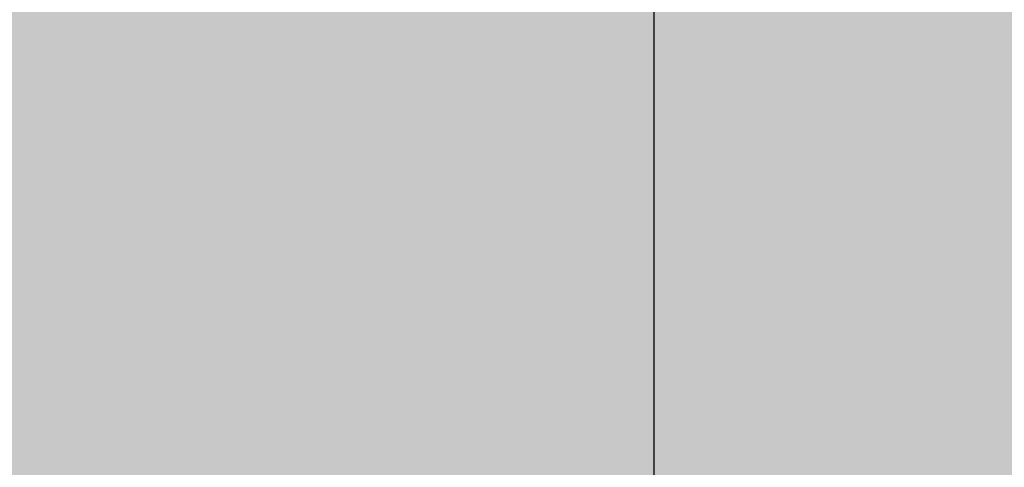
# Model space of a CAD drawing. Units: inches. Extents: x 2083 to 3317, y 1141 to 2115.
# Tile 46 of 256: x 2237.106 to 2238.294, y 1477.116 to 1477.656. Entities that reach past the tile are written whole.
import ezdxf

# ---------------------------------------------------------------- set-up
doc = ezdxf.new("R2010")
doc.units = ezdxf.units.IN
doc.layers.add('A-ANNO-DIMS', color=2, linetype='Continuous', lineweight=18)
doc.layers.add('A-WALL-PATT', color=251, linetype='Continuous', lineweight=13, true_color=0x636466)
doc.styles.get("Standard").update_dxf_attribs({"font": 'arial.ttf'})
doc.dimstyles.new('ISO-25', dxfattribs={"dimtxt": 12, "dimasz": 12, "dimexe": 1.25, "dimexo": 0.625, "dimtad": 1, "dimlunit": 3, "dimtxsty": 'Standard', "dimcen": 2.5, "dimadec": 0, "dimazin": 0, "dimtfac": 1, "dimtmove": 0, "dimatfit": 3, "dimfxl": 1, "dimarcsym": 0})

# ---------------------------------------------------------------- blocks, each defined once
blk = doc.blocks.new('*D30')
at = {"layer": 'A-ANNO-DIMS', "color": 0, "lineweight": -2, "transparency": 16777216}
for p, q in [((2240.0179, 1445.2738), (2240.0179, 1448.0455)), ((2254.3293, 1445.2738), (2254.3293, 1448.0455)), ((2228.0179, 1446.7955), (2216.0179, 1446.7955)), ((2240.0179, 1446.7955), (2254.3293, 1446.7955)), ((2266.3293, 1446.7955), (2413.7649, 1446.7955))]:
    blk.add_line(p, q, dxfattribs=at)
at = {"layer": 'A-ANNO-DIMS', "color": 0, "transparency": 16777216}
for points in [[(2228.0179, 1448.7955), (2228.0179, 1444.7955), (2240.0179, 1446.7955)], [(2266.3293, 1448.7955), (2266.3293, 1444.7955), (2254.3293, 1446.7955)]]:
    blk.add_solid(points, dxfattribs=at)
at = {"layer": 'Defpoints', "color": 0, "transparency": 16777216}
for p in [(2254.3293, 1446.7955), (2240.0179, 1444.6488), (2254.3293, 1444.6488)]:
    blk.add_point(p, dxfattribs=at)
at = {"layer": 'A-ANNO-DIMS', "color": 0, "transparency": 16777216, "insert": (2346.0471, 1453.6252), "char_height": 12, "attachment_point": 5}
blk.add_mtext('WC 1\'-2 1/2" TYP.', dxfattribs=at)
blk = doc.blocks.new('*D31')
at = {"layer": 'A-ANNO-DIMS', "color": 0, "lineweight": -2, "transparency": 16777216}
for p, q in [((2237.8711, 1456.6488), (2237.8711, 1541.9152)), ((2239.3929, 1444.6488), (2236.6211, 1444.6488)), ((2237.8711, 1431.5475), (2237.8711, 1444.6488)), ((2239.3929, 1431.5475), (2236.6211, 1431.5475)), ((2237.8711, 1419.5475), (2237.8711, 1407.5475))]:
    blk.add_line(p, q, dxfattribs=at)
at = {"layer": 'A-ANNO-DIMS', "color": 0, "transparency": 16777216}
for points in [[(2235.8711, 1456.6488), (2239.8711, 1456.6488), (2237.8711, 1444.6488)], [(2235.8711, 1419.5475), (2239.8711, 1419.5475), (2237.8711, 1431.5475)]]:
    blk.add_solid(points, dxfattribs=at)
at = {"layer": 'Defpoints', "color": 0, "transparency": 16777216}
for p in [(2237.8711, 1444.6488), (2240.0179, 1444.6488), (2240.0179, 1431.5475)]:
    blk.add_point(p, dxfattribs=at)
at = {"layer": 'A-ANNO-DIMS', "color": 0, "transparency": 16777216, "insert": (2231.2175, 1505.282), "char_height": 12, "attachment_point": 5, "rotation": 90}
blk.add_mtext('1\'-1" TYP.', dxfattribs=at)
blk = doc.blocks.new('*D62')
at = {"layer": 'A-ANNO-DIMS', "color": 0, "lineweight": -2, "transparency": 16777216}
for p, q in [((2235.9598, 1469.3864), (2235.9598, 1522.3614)), ((2379.9598, 1469.3864), (2379.9598, 1522.3614)), ((2247.9598, 1521.1114), (2367.9598, 1521.1114))]:
    blk.add_line(p, q, dxfattribs=at)
at = {"layer": 'A-ANNO-DIMS', "color": 0, "transparency": 16777216}
for points in [[(2247.9598, 1523.1114), (2247.9598, 1519.1114), (2235.9598, 1521.1114)], [(2367.9598, 1523.1114), (2367.9598, 1519.1114), (2379.9598, 1521.1114)]]:
    blk.add_solid(points, dxfattribs=at)
at = {"layer": 'Defpoints', "color": 0, "transparency": 16777216}
for p in [(2379.9598, 1521.1114), (2235.9598, 1468.7614), (2379.9598, 1468.7614)]:
    blk.add_point(p, dxfattribs=at)
at = {"layer": 'A-ANNO-DIMS', "color": 0, "transparency": 16777216, "insert": (2307.9598, 1527.8632), "char_height": 12, "attachment_point": 5}
blk.add_mtext('12\'-0"', dxfattribs=at)

msp = doc.modelspace()

# ---------------------------------------------------------------- hatches: boundary and pattern name
at = {"layer": 'A-WALL-PATT'}
h = msp.add_hatch(color=256, dxfattribs=at)
h.dxf.hatch_style = 1
h.paths.add_polyline_path([(3126.9598, 2020.7614), (2748.9598, 2020.7614), (2604.9598, 2020.7614), (2226.9598, 2020.7614), (2226.9598, 1702.7614), (2466.9598, 1702.7614), (2466.9598, 1582.7614), (2418.9598, 1582.7614), (2418.9598, 1477.7614), (2226.9598, 1477.7614), (2226.9598, 1263.2614), (2544.9598, 1263.2614), (2544.9598, 1411.7614), (2604.9598, 1411.7614), (2685.9598, 1411.7614), (2685.9598, 1420.7614), (2604.9598, 1420.7614), (2604.9598, 1573.7614), (2604.9598, 1702.7614), (2604.9598, 2011.7614), (2748.9598, 2011.7614), (2748.9598, 1702.7614), (2862.9598, 1702.7614), (2862.9598, 1621.7614), (2871.9598, 1621.7614), (2871.9598, 1702.7614), (2883.9598, 1702.7614), (2883.9598, 1706.9395, -0.026459), (2883.9598, 1711.7614), (2757.9598, 1711.7614), (2757.9598, 1807.7614), (2787.9598, 1807.7614), (2787.9598, 1812.2614), (2757.9598, 1812.2614), (2757.9598, 2011.7614), (2877.9598, 2011.7614), (2877.9598, 1812.2614), (2847.9598, 1812.2614), (2847.9598, 1807.7614), (2889.8357, 1807.7614), (2889.8357, 1812.2614), (2882.4598, 1812.2614), (2882.4598, 2011.7614), (3117.9598, 2011.7614), (3117.9598, 1812.2614), (2937.8357, 1812.2614), (2937.8357, 1807.7614), (2995.7098, 1807.7614), (2995.7098, 1796.1177), (3000.2098, 1796.1177), (3000.2098, 1807.7614), (3117.9598, 1807.7614), (3117.9598, 1711.7614), (3000.2098, 1711.7614), (3000.2098, 1760.1177), (2998.5727, 1760.1177, -0.020711), (2995.7098, 1760.1177), (2995.7098, 1711.7614), (2931.9598, 1711.7614), (2931.9598, 1702.7614), (3126.9598, 1702.7614)])
h.paths.add_polyline_path([(2471.4598, 2011.7614), (2471.4598, 1810.0114), (2462.7169, 1810.0114), (2462.7169, 1805.5114), (2505.9598, 1805.5114), (2505.9598, 1810.0114), (2475.9598, 1810.0114), (2475.9598, 2011.7614), (2595.9598, 2011.7614), (2595.9598, 1810.0114), (2565.9598, 1810.0114), (2565.9598, 1805.5114), (2595.9598, 1805.5114), (2595.9598, 1711.7614), (2235.9598, 1711.7614), (2235.9598, 1805.5114), (2353.7098, 1805.5114), (2353.7098, 1796.0542), (2358.2098, 1796.0542), (2358.2098, 1805.5114), (2414.7169, 1805.5114), (2414.7169, 1810.0114), (2235.9598, 1810.0114), (2235.9598, 2011.7614)], flags=16)
h.paths.add_polyline_path([(2270.2047, 1994.61), (2270.2047, 1970.61), (2246.2047, 1970.61), (2246.2047, 1994.61)], flags=0)
edge = h.paths.add_edge_path(flags=0)
edge.add_ellipse((2332.0274, 1899.7982), major_axis=(-3.043, 3.043), ratio=0.168252, start_angle=-161.3322, end_angle=-156.3071, ccw=False)
edge.add_ellipse((2333.082, 1898.7435), major_axis=(-1.0546, 1.0546), ratio=0.453532, start_angle=-123.371, end_angle=-94.1591)
edge = h.paths.add_edge_path(flags=0)
edge.add_ellipse((2332.0274, 1968.8763), major_axis=(3.043, 3.043), ratio=0.168252, start_angle=18.6678, end_angle=23.6929)
edge.add_spline(control_points=[(2332.9256, 1970.6911), (2332.2268, 1970.3361), (2330.8937, 1969.6589), (2328.4131, 1970.9321), (2327.2039, 1967.7487), (2324.7096, 1969.9556), (2322.5328, 1967.0124), (2320.0128, 1971.2958), (2317.6803, 1968.1578), (2316.0405, 1967.102), (2315.4269, 1966.8096)], knot_values=[0, 0, 0, 0, 2.267059, 4.324559, 6.685584, 8.878641, 11.121502, 14.300359, 17.755284, 19.732645, 19.732645, 19.732645, 19.732645], degree=3, periodic=0)
edge.add_ellipse((2332.0274, 1968.8763), major_axis=(3.043, 3.043), ratio=0.168252, start_angle=18.6678, end_angle=23.6929, ccw=False)
edge.add_ellipse((2333.082, 1969.9309), major_axis=(1.0546, 1.0546), ratio=0.453532, start_angle=56.629, end_angle=85.8409, ccw=False)
edge = h.paths.add_edge_path(flags=0)
edge.add_spline(control_points=[(2296.4283, 1967.9879), (2293.6278, 1965.3363), (2287.7036, 1959.7271), (2299.7439, 1949.9957), (2294.5326, 1935.6685), (2290.5732, 1920.6035), (2293.3941, 1909.9737), (2296.1854, 1904.9665)], knot_values=[0.099185, 0.099185, 0.099185, 0.099185, 0.345301, 0.619822, 0.982653, 1.386093, 1.810555, 1.810555, 1.810555, 1.810555], degree=3, periodic=0)
edge.add_spline(control_points=[(2296.1854, 1904.9665), (2297.3836, 1902.6193), (2298.001, 1901.9493), (2298.553, 1901.4682)], knot_values=[0.006246, 0.006246, 0.006246, 0.006246, 0.055476, 0.055476, 0.055476, 0.055476], degree=3, periodic=0)
edge.add_spline(control_points=[(2298.553, 1901.4682), (2297.2586, 1900.9232), (2295.2253, 1900.2321), (2293.0602, 1900.6142), (2292.1014, 1900.7884), (2292.0896, 1900.7906)], knot_values=[0.312835, 0.312835, 0.312835, 0.312835, 0.40178, 0.474987, 0.475903, 0.475903, 0.475903, 0.475903], degree=3, periodic=0)
edge.add_arc((2292.7936, 1904.6641), 3.937, 215.4209, 259.6982, ccw=False)
edge.add_spline(control_points=[(2289.5853, 1902.3823), (2289.4767, 1902.5351), (2289.3685, 1902.688), (2289.2609, 1902.8412)], knot_values=[0.102872, 0.102872, 0.102872, 0.102872, 0.116896, 0.116896, 0.116896, 0.116896], degree=3, periodic=0)
edge.add_spline(control_points=[(2289.2609, 1902.8412), (2288.6866, 1902.5502), (2287.64, 1902.0199), (2285.8813, 1901.874), (2283.853, 1901.5044), (2281.72, 1899.7105), (2278.467, 1899.4929), (2276.1571, 1901.8832), (2272.259, 1899.8041), (2267.7776, 1901.8432), (2262.2439, 1900.184), (2257.4149, 1901.7821), (2254.3184, 1900.7261), (2253.1783, 1900.3373)], knot_values=[0, 0, 0, 0, 1.907977, 3.477176, 5.261074, 7.972851, 11.680248, 13.717921, 16.939592, 22.789562, 27.502503, 33.595215, 37.145618, 37.145618, 37.145618, 37.145618], degree=3, periodic=0)
edge.add_line((2253.1783, 1900.3373), (2250.2442, 1902.8412))
edge.add_line((2250.2442, 1902.8412), (2250.2442, 1965.8333))
edge.add_line((2250.2442, 1965.8333), (2253.1783, 1968.3371))
edge.add_spline(control_points=[(2253.1783, 1968.3371), (2254.3184, 1967.9483), (2257.4149, 1966.8924), (2262.2439, 1968.4904), (2267.7776, 1966.8313), (2271.5267, 1968.5372), (2273.8759, 1967.8283), (2274.2067, 1967.7276)], knot_values=[0, 0, 0, 0, 0.09018, 0.244935, 0.364644, 0.513233, 0.537855, 0.537855, 0.537855, 0.537855], degree=3, periodic=0)
edge.add_arc((2274.3529, 1963.7933), 3.937, 72.0511, 92.1279, ccw=False)
edge.add_arc((2281.2969, 1985.23), 18.5963, 252.05113, 288.56572)
edge.add_arc((2292.3167, 1956.0289), 12.6461, 71.02679, 113.77822, ccw=False)
edge = h.paths.add_edge_path(flags=0)
edge.add_spline(control_points=[(2274.8994, 1951.8562), (2275.0662, 1951.6166), (2275.2327, 1951.3766), (2275.398, 1951.1359)], knot_values=[1.409916, 1.409916, 1.409916, 1.409916, 1.43159, 1.43159, 1.43159, 1.43159], degree=3, periodic=0)
edge.add_spline(control_points=[(2275.398, 1951.1359), (2275.7921, 1950.5619), (2276.1792, 1949.9838), (2276.5455, 1949.3971)], knot_values=[1.358238, 1.358238, 1.358238, 1.358238, 1.409916, 1.409916, 1.409916, 1.409916], degree=3, periodic=0)
edge.add_line((2276.5455, 1949.3971), (2277.4373, 1947.8622))
edge.add_spline(control_points=[(2277.4373, 1947.8622), (2276.3038, 1945.6731), (2274.6397, 1942.4269), (2274.6316, 1938.0939), (2272.7991, 1930.8515), (2274.3564, 1943.897), (2275.9477, 1947.9234), (2276.5455, 1949.3971)], knot_values=[0.005632, 0.005632, 0.005632, 0.005632, 0.186014, 0.266002, 0.357087, 0.59639, 0.739732, 0.739732, 0.739732, 0.739732], degree=3, periodic=0)
edge.add_spline(control_points=[(2276.5455, 1949.3971), (2276.1792, 1949.9838), (2275.7921, 1950.5619), (2275.398, 1951.1359)], knot_values=[1.358238, 1.358238, 1.358238, 1.358238, 1.409916, 1.409916, 1.409916, 1.409916], degree=3, periodic=0)
edge.add_spline(control_points=[(2275.398, 1951.1359), (2274.9425, 1950.0805), (2274.2078, 1948.0253), (2273.9346, 1944.8515), (2272.4685, 1937.6275), (2273.4662, 1945.6965), (2274.7006, 1951.0595), (2274.8994, 1951.8562)], knot_values=[0.104364, 0.104364, 0.104364, 0.104364, 0.189636, 0.269624, 0.36071, 0.600013, 0.644622, 0.644622, 0.644622, 0.644622], degree=3, periodic=0)
h.paths.add_polyline_path([(2269.1675, 1963.1276, -0.357527), (2268.1706, 1960.9764, -0.092561), (2268.1706, 1939.4363, -0.357527), (2269.1675, 1937.2851, -0.357527), (2267.0163, 1938.282, -0.164785), (2254.6856, 1938.282, -0.357527), (2252.5344, 1937.2851, -0.357527), (2253.5313, 1939.4363, -0.092561), (2253.5313, 1960.9764, -0.357527), (2252.5344, 1963.1276, -0.357527), (2254.6856, 1962.1307, -0.164785), (2267.0163, 1962.1307, -0.357527)], flags=0)
h.paths.add_polyline_path([(2248.8741, 1967.8018), (2248.8741, 1957.0277), (2249.4578, 1957.0277), (2249.4578, 1911.6468), (2248.8741, 1911.6468), (2248.8741, 1900.8727), (2246.5119, 1900.8727, 0.197327), (2244.1497, 1902.4569), (2244.1497, 1966.2176, 0.197327), (2246.5119, 1967.8018)], flags=0)
h.paths.add_polyline_path([(2269.1675, 1931.3893, -0.357527), (2268.1706, 1929.2381, -0.092561), (2268.1706, 1907.6981, -0.357527), (2269.1675, 1905.5469, -0.357527), (2267.0163, 1906.5438, -0.164785), (2254.6856, 1906.5438, -0.357527), (2252.5344, 1905.5469, -0.357527), (2253.5313, 1907.6981, -0.092561), (2253.5313, 1929.2381, -0.357527), (2252.5344, 1931.3893, -0.357527), (2254.6856, 1930.3925, -0.164785), (2267.0163, 1930.3925, -0.357527)], flags=0)
edge = h.paths.add_edge_path(flags=0)
edge.add_spline(control_points=[(2276.1969, 1906.7237), (2276.1681, 1909.0289), (2276.114, 1913.3719), (2270.5984, 1924.925), (2273.9052, 1919.0128), (2275.9217, 1916.2621), (2275.4746, 1912.4021), (2277.2579, 1910.3806), (2276.696, 1908.225), (2276.6462, 1906.813), (2276.6178, 1906.0084)], knot_values=[0, 0, 0, 0, 8.61026, 16.221274, 18.843057, 23.804898, 27.440828, 29.356102, 31.203478, 33.650687, 33.650687, 33.650687, 33.650687], degree=3, periodic=0)
edge.add_spline(control_points=[(2276.6178, 1906.0084), (2276.6233, 1905.6241), (2276.4977, 1904.6287), (2275.4418, 1903.8547), (2274.9373, 1903.0804), (2274.8591, 1902.8412)], knot_values=[0.156488, 0.156488, 0.156488, 0.156488, 0.184398, 0.231376, 0.250598, 0.250598, 0.250598, 0.250598], degree=3, periodic=0)
edge.add_line((2274.8591, 1902.8412), (2276.506, 1902.8412))
edge.add_spline(control_points=[(2276.506, 1902.8412), (2276.7883, 1903.0849), (2277.6651, 1904.1252), (2278.2495, 1904.3407), (2277.6539, 1908.5274), (2278.1557, 1906.2278), (2278.1005, 1905.2859), (2278.8467, 1904.069), (2277.8568, 1903.4149), (2277.8742, 1902.991), (2277.9036, 1902.8412)], knot_values=[0.059574, 0.059574, 0.059574, 0.059574, 0.080753, 0.103741, 0.16972, 0.176036, 0.207137, 0.240474, 0.262341, 0.27366, 0.27366, 0.27366, 0.27366], degree=3, periodic=0)
edge.add_line((2277.9036, 1902.8412), (2280.0298, 1902.8412))
edge.add_spline(control_points=[(2280.0298, 1902.8412), (2279.8882, 1903.0884), (2279.4993, 1903.9816), (2280.1523, 1905.9393), (2278.1036, 1909.6578), (2279.7624, 1907.1853), (2280.3279, 1904.8749), (2280.4851, 1903.4896), (2281.4633, 1903.2494), (2281.7583, 1902.9365), (2281.834, 1902.8412)], knot_values=[0.013856, 0.013856, 0.013856, 0.013856, 0.034874, 0.088867, 0.107879, 0.126738, 0.158714, 0.193757, 0.217487, 0.226722, 0.226722, 0.226722, 0.226722], degree=3, periodic=0)
edge.add_spline(control_points=[(2281.834, 1902.8412), (2281.7875, 1902.8267), (2281.647, 1902.783), (2281.3955, 1902.8595), (2281.0881, 1902.9852), (2280.7207, 1903.0609), (2280.3335, 1903.0257), (2280.1248, 1902.8989), (2280.0298, 1902.8412)], knot_values=[0, 0, 0, 0, 0.14413, 0.435517, 0.749276, 1.153046, 1.548371, 1.878348, 1.878348, 1.878348, 1.878348], degree=3, periodic=0)
edge.add_line((2280.0298, 1902.8412), (2277.9036, 1902.8412))
edge.add_spline(control_points=[(2277.9036, 1902.8412), (2277.8929, 1902.7959), (2277.8654, 1902.6796), (2277.6075, 1902.6875), (2277.2741, 1902.8007), (2276.8379, 1902.6198), (2276.5838, 1902.7893), (2276.506, 1902.8412)], knot_values=[0, 0, 0, 0, 0.127189, 0.326199, 0.628009, 1.24357, 1.515331, 1.515331, 1.515331, 1.515331], degree=3, periodic=0)
edge.add_line((2276.506, 1902.8412), (2274.8591, 1902.8412))
edge.add_spline(control_points=[(2274.8591, 1902.8412), (2274.8144, 1902.8986), (2274.7251, 1903.0134), (2274.4935, 1903.119), (2274.2443, 1902.9605), (2273.9371, 1903.1849), (2273.614, 1902.9831), (2273.4083, 1902.883), (2273.3223, 1902.8412)], knot_values=[0, 0, 0, 0, 0.21843, 0.436957, 0.687977, 0.990379, 1.398396, 1.69185, 1.69185, 1.69185, 1.69185], degree=3, periodic=0)
edge.add_spline(control_points=[(2273.3223, 1902.8412), (2273.6167, 1903.4457), (2274.274, 1904.5383), (2276.0272, 1904.5737), (2276.207, 1906.5836), (2276.1969, 1906.7237)], knot_values=[0.012227, 0.012227, 0.012227, 0.012227, 0.059472, 0.106218, 0.134458, 0.134458, 0.134458, 0.134458], degree=3, periodic=0)
h.paths.add_polyline_path([(2270.7761, 1897.7898), (2270.7761, 1873.7898), (2246.7761, 1873.7898), (2246.7761, 1897.7898)], flags=0)
h.paths.add_polyline_path([(2353.7098, 1760.0051), (2353.7098, 1760.0542), (2358.2098, 1760.0542, -0.033729)], flags=0)
h.paths.add_polyline_path([(2321.8191, 1737.5292), (2341.9953, 1737.5292, -0.414214), (2343.2033, 1736.3212), (2343.2033, 1721.0206, -0.414214), (2341.9953, 1719.8127), (2321.8191, 1719.8127, -0.414214), (2320.6112, 1721.0206), (2320.6112, 1736.3212, -0.414214)], flags=0)
h.paths.add_polyline_path([(2324.235, 1736.3212), (2339.5794, 1736.3212, -0.414214), (2341.9953, 1733.9053), (2341.9953, 1725.4497, -0.414214), (2339.5794, 1723.0338), (2333.6806, 1723.0338), (2333.8453, 1722.0455, -0.870646), (2335.4254, 1721.8259, -0.767327), (2333.9227, 1721.4232), (2331.291, 1721.4232, -0.767327), (2329.7883, 1721.8259, -0.870646), (2331.3684, 1722.0455), (2331.5331, 1723.0338), (2324.235, 1723.0338, -0.414214), (2321.8191, 1725.4497), (2321.8191, 1733.9053, -0.414214)], flags=0)
h.paths.add_polyline_path([(2570.4838, 1928.6154), (2589.6838, 1928.6154), (2590.1688, 1928.6154), (2590.1688, 1904.9934), (2570.4838, 1904.9934)], flags=0)
h.paths.add_polyline_path([(2574.4473, 1927.2638, -1), (2572.8288, 1927.2638, -1)], flags=0)
h.paths.add_polyline_path([(2573.0899, 1926.9409), (2573.925, 1927.776), (2574.1477, 1927.5533), (2573.3126, 1926.7182)], flags=0)
h.paths.add_polyline_path([(2578.7791, 1919.7296, -1), (2571.5917, 1919.7296, -1)], flags=0)
h.paths.add_polyline_path([(2578.3854, 1919.7296, -1), (2571.9854, 1919.7296, -1)], flags=0)
h.paths.add_polyline_path([(2331.5958, 1729.4762, -1), (2333.618, 1729.4762, -1)], flags=0)
h.paths.add_polyline_path([(2578.0342, 1927.2638, -1), (2576.4157, 1927.2638, -1)], flags=0)
h.paths.add_polyline_path([(2576.6889, 1927.5311), (2576.9116, 1927.7538), (2577.7467, 1926.9186), (2577.524, 1926.6959)], flags=0)
h.paths.add_polyline_path([(2578.1391, 1909.8595, -1), (2572.2317, 1909.8595, -1)], flags=0)
h.paths.add_polyline_path([(2577.7454, 1909.8595, -1), (2572.6254, 1909.8595, -1)], flags=0)
h.paths.add_polyline_path([(2583.7977, 1927.2638, -1), (2582.1792, 1927.2638, -1)], flags=0)
h.paths.add_polyline_path([(2582.7186, 1927.7538), (2583.5538, 1926.9186), (2583.3311, 1926.6959), (2582.4959, 1927.5311)], flags=0)
h.paths.add_polyline_path([(2582.4959, 1927.5311), (2582.7186, 1927.7538), (2583.5538, 1926.9186), (2583.3311, 1926.6959)], flags=0)
h.paths.add_polyline_path([(2587.7391, 1920.5296, -1), (2581.8317, 1920.5296, -1)], flags=0)
h.paths.add_polyline_path([(2587.3454, 1920.5296, -1), (2582.2254, 1920.5296, -1)], flags=0)
h.paths.add_polyline_path([(2587.3846, 1927.2638, -1), (2585.7661, 1927.2638, -1)], flags=0)
h.paths.add_polyline_path([(2586.082, 1926.9802), (2586.9172, 1927.8154), (2587.1399, 1927.5927), (2586.3047, 1926.7575)], flags=0)
h.paths.add_polyline_path([(2588.3791, 1910.6595, -1), (2581.1917, 1910.6595, -1)], flags=0)
h.paths.add_polyline_path([(2587.9854, 1910.6595, -1), (2581.5854, 1910.6595, -1)], flags=0)
h.paths.add_polyline_path([(2417.1677, 1729.4779), (2437.3439, 1729.4779, -0.414214), (2438.5519, 1728.2699), (2438.5519, 1712.9693, -0.414214), (2437.3439, 1711.7614), (2417.1677, 1711.7614, -0.414214), (2415.9598, 1712.9693), (2415.9598, 1728.2699, -0.414214)], flags=0)
h.paths.add_polyline_path([(2419.5836, 1728.2699), (2434.928, 1728.2699, -0.414214), (2437.3439, 1725.8541), (2437.3439, 1717.3984, -0.414214), (2434.928, 1714.9825), (2429.0292, 1714.9825), (2429.1939, 1713.9942, -0.870646), (2430.774, 1713.7746, -0.767327), (2429.2713, 1713.372), (2426.6396, 1713.372, -0.767327), (2425.1369, 1713.7746, -0.870646), (2426.717, 1713.9942), (2426.8817, 1714.9825), (2419.5836, 1714.9825, -0.414214), (2417.1677, 1717.3984), (2417.1677, 1725.8541, -0.414214)], flags=0)
h.paths.add_polyline_path([(2419.5836, 1728.2699), (2434.928, 1728.2699, -0.414214), (2437.3439, 1725.8541), (2437.3439, 1717.3984, -0.414214), (2434.928, 1714.9825), (2429.0292, 1714.9825), (2428.3581, 1719.009), (2427.5528, 1719.009), (2426.8817, 1714.9825), (2419.5836, 1714.9825, -0.414214), (2417.1677, 1717.3984), (2417.1677, 1725.8541, -0.414214)], flags=0)
h.paths.add_polyline_path([(2426.9444, 1721.4249, -1), (2428.9666, 1721.4249, -1)], flags=0)
h.paths.add_polyline_path([(2475.9598, 1702.7614), (2595.9598, 1702.7614), (2595.9598, 1582.7614), (2475.9598, 1582.7614)], flags=16)
h.paths.add_polyline_path([(2427.9598, 1573.7614), (2595.9598, 1573.7614), (2595.9598, 1468.7614), (2595.9598, 1420.7614), (2384.4598, 1420.7614), (2384.4598, 1468.7614), (2427.9598, 1468.7614)], flags=16)
h.paths.add_polyline_path([(2379.9598, 1468.7614), (2379.9598, 1420.7614), (2235.9598, 1420.7614), (2235.9598, 1468.7614)], flags=16)
h.paths.add_polyline_path([(2317.816, 1466.6958), (2337.9922, 1466.6958, -0.414214), (2339.2002, 1465.4878), (2339.2002, 1450.1872, -0.414214), (2337.9922, 1448.9792), (2317.816, 1448.9792, -0.414214), (2316.6081, 1450.1872), (2316.6081, 1465.4878, -0.414214)], flags=0)
h.paths.add_polyline_path([(2320.2319, 1465.4878), (2335.5763, 1465.4878, -0.414214), (2337.9922, 1463.0719), (2337.9922, 1454.6163, -0.414214), (2335.5763, 1452.2004), (2329.6775, 1452.2004), (2329.8422, 1451.212, -0.870646), (2331.4223, 1450.9925, -0.767327), (2329.9196, 1450.5898), (2327.2879, 1450.5898, -0.767327), (2325.7852, 1450.9925, -0.870646), (2327.3653, 1451.212), (2327.53, 1452.2004), (2320.2319, 1452.2004, -0.414214), (2317.816, 1454.6163), (2317.816, 1463.0719, -0.414214)], flags=0)
h.paths.add_polyline_path([(2320.2319, 1465.4878), (2335.5763, 1465.4878, -0.414214), (2337.9922, 1463.0719), (2337.9922, 1454.6163, -0.414214), (2335.5763, 1452.2004), (2329.6775, 1452.2004), (2329.0064, 1456.2269), (2328.2011, 1456.2269), (2327.53, 1452.2004), (2320.2319, 1452.2004, -0.414214), (2317.816, 1454.6163), (2317.816, 1463.0719, -0.414214)], flags=0)
h.paths.add_polyline_path([(2327.5926, 1458.6428, -1), (2329.6148, 1458.6428, -1)], flags=0)
h.paths.add_polyline_path([(2244.4117, 1433.3405), (2241.9209, 1433.3405, -0.414214), (2240.0179, 1435.2435), (2240.0179, 1440.9528, -0.414211), (2241.9209, 1442.8559), (2244.4117, 1442.8559, -1.976472)], flags=0)
h.paths.add_polyline_path([(2245.3569, 1434.3975, -0.414214), (2245.3569, 1441.7988, -2.144098)], flags=0)
h.paths.add_polyline_path([(2535.9598, 1416.2614), (2535.9598, 1272.2614), (2235.9598, 1272.2614), (2235.9598, 1416.2614)], flags=16)
h.paths.add_polyline_path([(2260.1196, 1384.2928), (2260.1196, 1362.0386), (2237.8654, 1362.0386), (2237.8654, 1384.2928)], flags=0)
edge = h.paths.add_edge_path(flags=0)
edge.add_line((2318.2518, 1362.0933), (2318.1458, 1362.001))
edge.add_ellipse((2317.4451, 1360.431), major_axis=(2.8216, 2.8216), ratio=0.168252, start_angle=18.6678, end_angle=20.9481, ccw=False)
edge.add_ellipse((2318.423, 1361.409), major_axis=(0.9779, 0.9779), ratio=0.453532, start_angle=56.629, end_angle=70.2262, ccw=False)
edge = h.paths.add_edge_path(flags=0)
edge.add_line((2319.1074, 1295.5711), (2319.015, 1295.6771))
edge.add_ellipse((2317.4451, 1296.3778), major_axis=(-2.8216, 2.8216), ratio=0.168252, start_angle=-161.3322, end_angle=-159.0519, ccw=False)
edge.add_ellipse((2318.423, 1295.3999), major_axis=(-0.9779, 0.9779), ratio=0.453532, start_angle=-123.371, end_angle=-109.7738)
edge = h.paths.add_edge_path(flags=0)
edge.add_spline(control_points=[(2284.2103, 1301.1702), (2284.5807, 1300.4447), (2284.8912, 1299.892), (2285.1596, 1299.461)], knot_values=[0.039066, 0.039066, 0.039066, 0.039066, 0.055476, 0.055476, 0.055476, 0.055476], degree=3, periodic=0)
edge.add_line((2285.1596, 1299.461), (2284.2103, 1301.1702))
edge = h.paths.add_edge_path(flags=0)
edge.add_line((2280.4125, 1297.298), (2283.37, 1297.0361))
edge.add_line((2283.37, 1297.0361), (2286.4057, 1297.9263))
edge.add_spline(control_points=[(2286.4057, 1297.9263), (2285.3055, 1297.4631), (2284.3448, 1297.1292), (2283.37, 1297.0361)], knot_values=[0.394369, 0.394369, 0.394369, 0.394369, 0.475903, 0.475903, 0.475903, 0.475903], degree=3, periodic=0)
edge.add_spline(control_points=[(2283.37, 1297.0361), (2283.2814, 1297.0277), (2282.3163, 1296.9573), (2281.3125, 1297.1345), (2280.4234, 1297.296), (2280.4125, 1297.298)], knot_values=[0.312835, 0.312835, 0.312835, 0.312835, 0.320246, 0.393453, 0.394369, 0.394369, 0.394369, 0.394369], degree=3, periodic=0)
edge = h.paths.add_edge_path(flags=0)
edge.add_line((2284.4356, 1359.6073), (2280.4463, 1355.328))
edge.add_line((2280.4463, 1355.328), (2279.58, 1351.0178))
edge.add_line((2279.58, 1351.0178), (2282.413, 1346.5804))
edge.add_spline(control_points=[(2282.413, 1346.5804), (2283.1533, 1345.5892), (2284.2529, 1344.0289), (2284.801, 1342.3872), (2284.9352, 1341.8055)], knot_values=[1.240098, 1.240098, 1.240098, 1.240098, 1.332892, 1.382712, 1.382712, 1.382712, 1.382712], degree=3, periodic=0)
edge.add_spline(control_points=[(2284.9352, 1341.8055), (2285.3191, 1340.1406), (2285.233, 1338.4092), (2284.9099, 1336.6541)], knot_values=[1.097484, 1.097484, 1.097484, 1.097484, 1.240098, 1.240098, 1.240098, 1.240098], degree=3, periodic=0)
edge.add_spline(control_points=[(2284.9099, 1336.6541), (2284.5868, 1334.899), (2284.0267, 1333.1203), (2283.4626, 1331.3606)], knot_values=[0.95487, 0.95487, 0.95487, 0.95487, 1.097484, 1.097484, 1.097484, 1.097484], degree=3, periodic=0)
edge.add_line((2283.4626, 1331.3606), (2281.8904, 1326.1534))
edge.add_line((2281.8904, 1326.1534), (2280.7563, 1321.0561))
edge.add_line((2280.7563, 1321.0561), (2280.2992, 1316.002))
edge.add_line((2280.2992, 1316.002), (2280.7159, 1310.9501))
edge.add_line((2280.7159, 1310.9501), (2282.0281, 1305.9721))
edge.add_line((2282.0281, 1305.9721), (2284.2103, 1301.1702))
edge.add_spline(control_points=[(2284.2103, 1301.1702), (2283.3407, 1302.7302), (2282.6119, 1304.3365), (2282.0281, 1305.9721)], knot_values=[0.099185, 0.099185, 0.099185, 0.099185, 0.241799, 0.241799, 0.241799, 0.241799], degree=3, periodic=0)
edge.add_spline(control_points=[(2282.0281, 1305.9721), (2281.4443, 1307.6078), (2281.0055, 1309.2728), (2280.7159, 1310.9501)], knot_values=[0.241799, 0.241799, 0.241799, 0.241799, 0.384413, 0.384413, 0.384413, 0.384413], degree=3, periodic=0)
edge.add_spline(control_points=[(2280.7159, 1310.9501), (2280.4332, 1312.5876), (2280.2894, 1314.277), (2280.2989, 1315.962), (2280.2992, 1316.002)], knot_values=[0.384413, 0.384413, 0.384413, 0.384413, 0.523647, 0.527028, 0.527028, 0.527028, 0.527028], degree=3, periodic=0)
edge.add_spline(control_points=[(2280.2992, 1316.002), (2280.3123, 1317.687), (2280.4779, 1319.3679), (2280.7563, 1321.0561)], knot_values=[0.527028, 0.527028, 0.527028, 0.527028, 0.669642, 0.669642, 0.669642, 0.669642], degree=3, periodic=0)
edge.add_spline(control_points=[(2280.7563, 1321.0561), (2281.0346, 1322.7443), (2281.4259, 1324.4396), (2281.8904, 1326.1534)], knot_values=[0.669642, 0.669642, 0.669642, 0.669642, 0.812256, 0.812256, 0.812256, 0.812256], degree=3, periodic=0)
edge.add_spline(control_points=[(2281.8904, 1326.1534), (2282.2644, 1327.5333), (2282.7879, 1329.2618), (2283.3528, 1331.0178), (2283.4626, 1331.3606)], knot_values=[0.812256, 0.812256, 0.812256, 0.812256, 0.927087, 0.95487, 0.95487, 0.95487, 0.95487], degree=3, periodic=0)
edge.add_line((2283.4626, 1331.3606), (2284.9099, 1336.6541))
edge.add_line((2284.9099, 1336.6541), (2284.9352, 1341.8055))
edge.add_line((2284.9352, 1341.8055), (2282.413, 1346.5804))
edge.add_spline(control_points=[(2282.413, 1346.5804), (2281.2751, 1348.1038), (2280.0784, 1349.5703), (2279.58, 1351.0178)], knot_values=[1.382712, 1.382712, 1.382712, 1.382712, 1.525326, 1.525326, 1.525326, 1.525326], degree=3, periodic=0)
edge.add_spline(control_points=[(2279.58, 1351.0178), (2279.4433, 1351.4147), (2279.1363, 1352.8569), (2279.7352, 1354.2904), (2280.4463, 1355.328)], knot_values=[1.525326, 1.525326, 1.525326, 1.525326, 1.564439, 1.667941, 1.667941, 1.667941, 1.667941], degree=3, periodic=0)
edge.add_spline(control_points=[(2280.4463, 1355.328), (2281.4261, 1356.7578), (2282.9308, 1358.1826), (2284.4356, 1359.6073)], knot_values=[1.667941, 1.667941, 1.667941, 1.667941, 1.810555, 1.810555, 1.810555, 1.810555], degree=3, periodic=0)
edge.add_arc((2280.6231, 1348.5182), 11.7262, 71.02679, 113.77822)
edge.add_arc((2270.4049, 1375.5952), 17.2436, 252.05113, 288.56572, ccw=False)
edge.add_arc((2263.966, 1355.7178), 3.6506, 72.0511, 92.1279)
edge.add_arc((2263.966, 1355.7178), 3.6506, 92.1279, 177.9851)
edge.add_spline(control_points=[(2260.3176, 1355.8462), (2260.2604, 1354.2207), (2260.5513, 1350.1865), (2262.9993, 1346.7663), (2264.4727, 1344.649)], knot_values=[1.43159, 1.43159, 1.43159, 1.43159, 1.564144, 1.770695, 1.770695, 1.770695, 1.770695], degree=3, periodic=0)
edge.add_line((2264.4727, 1344.649), (2264.9356, 1343.9825))
edge.add_spline(control_points=[(2263.801, 1340.2481), (2263.8432, 1340.5141), (2264.0672, 1341.7565), (2264.5127, 1343.0025), (2264.935, 1343.9811)], knot_values=[0.53657, 0.53657, 0.53657, 0.53657, 0.559349, 0.644622, 0.644622, 0.644622, 0.644622], degree=3, periodic=0)
edge.add_spline(control_points=[(2264.935, 1343.9811), (2265.1178, 1343.715), (2265.2989, 1343.4479), (2265.4768, 1343.1794)], knot_values=[1.384077, 1.384077, 1.384077, 1.384077, 1.409916, 1.409916, 1.409916, 1.409916], degree=3, periodic=0)
edge.add_spline(control_points=[(2265.4768, 1343.1794), (2265.6546, 1342.9108), (2265.8293, 1342.6408), (2265.9991, 1342.3688)], knot_values=[1.358238, 1.358238, 1.358238, 1.358238, 1.384077, 1.384077, 1.384077, 1.384077], degree=3, periodic=0)
edge.add_line((2265.9991, 1342.3688), (2266.826, 1340.9455))
edge.add_spline(control_points=[(2266.826, 1340.9455), (2268.8944, 1337.0897), (2271.3982, 1325.843), (2270.5162, 1310.5686), (2275.9194, 1301.8606), (2277.7895, 1299.1994)], knot_values=[0.116896, 0.116896, 0.116896, 0.116896, 0.472987, 1.050969, 1.313793, 1.313793, 1.313793, 1.313793], degree=3, periodic=0)
edge.add_spline(control_points=[(2277.7895, 1299.1994), (2277.8394, 1299.1285), (2277.8894, 1299.0575), (2277.9396, 1298.9866)], knot_values=[0.109884, 0.109884, 0.109884, 0.109884, 0.116896, 0.116896, 0.116896, 0.116896], degree=3, periodic=0)
edge.add_line((2277.9396, 1298.9866), (2277.7888, 1299.1991))
edge.add_spline(control_points=[(2277.7888, 1299.1991), (2277.2566, 1298.9294), (2276.2864, 1298.4379), (2275.0394, 1298.3344), (2274.3833, 1298.2389), (2274.2153, 1298.2093)], knot_values=[33.12187, 33.12187, 33.12187, 33.12187, 35.029056, 36.598255, 37.144827, 37.144827, 37.144827, 37.144827], degree=3, periodic=0)
edge.add_line((2274.2153, 1298.2093), (2273.0731, 1297.893))
edge.add_spline(control_points=[(2273.0731, 1297.893), (2272.3229, 1297.5798), (2271.0392, 1296.5105), (2269.2484, 1296.2261), (2268.4231, 1296.3747)], knot_values=[26.532584, 26.532584, 26.532584, 26.532584, 29.198919, 31.839101, 31.839101, 31.839101, 31.839101], degree=3, periodic=0)
edge.add_line((2268.4231, 1296.3747), (2263.8785, 1297.4575))
edge.add_spline(control_points=[(2263.8785, 1297.4575), (2263.5561, 1297.3594), (2261.8603, 1296.8387), (2260.2388, 1297.2824), (2258.9335, 1297.5165)], knot_values=[15.919551, 15.919551, 15.919551, 15.919551, 16.939592, 21.226067, 21.226067, 21.226067, 21.226067], degree=3, periodic=0)
edge.add_line((2258.9335, 1297.5165), (2254.0552, 1297.329))
edge.add_spline(control_points=[(2254.0552, 1297.329), (2253.7555, 1297.2958), (2252.1137, 1297.1652), (2250.4619, 1297.5442), (2249.1297, 1297.6679)], knot_values=[5.306517, 5.306517, 5.306517, 5.306517, 6.276435, 10.613034, 10.613034, 10.613034, 10.613034], degree=3, periodic=0)
edge.add_line((2249.1297, 1297.6679), (2244.3316, 1296.8778))
edge.add_line((2244.3316, 1296.8778), (2241.611, 1299.1994))
edge.add_line((2241.611, 1299.1994), (2241.611, 1357.6094))
edge.add_line((2241.611, 1357.6094), (2244.3316, 1359.9311))
edge.add_line((2244.3316, 1359.9311), (2252.7288, 1359.5427))
edge.add_spline(control_points=[(2252.7288, 1359.5427), (2252.8709, 1359.5464), (2253.3057, 1359.5482), (2253.7398, 1359.5143), (2254.0317, 1359.4824)], knot_values=[0.233291, 0.233291, 0.233291, 0.233291, 0.244935, 0.268927, 0.268927, 0.268927, 0.268927], degree=3, periodic=0)
edge.add_line((2254.0317, 1359.4824), (2259.5872, 1359.4164))
edge.add_spline(control_points=[(2259.5872, 1359.4164), (2260.6771, 1359.6285), (2262.0732, 1359.897), (2263.5237, 1359.4593), (2263.8304, 1359.366)], knot_values=[0.422516, 0.422516, 0.422516, 0.422516, 0.513233, 0.537855, 0.537855, 0.537855, 0.537855], degree=3, periodic=0)
edge.add_arc((2263.966, 1355.7178), 3.6506, 72.0511, 92.1279, ccw=False)
edge.add_arc((2270.4049, 1375.5952), 17.2436, 252.05113, 288.56572)
edge.add_arc((2280.6231, 1348.5182), 11.7262, 71.02679, 113.77822, ccw=False)
h.paths.add_polyline_path([(2240.3405, 1359.4347), (2240.3405, 1349.4444), (2240.8818, 1349.4444), (2240.8818, 1307.3645), (2240.3405, 1307.3645), (2240.3405, 1297.3741), (2238.1502, 1297.3741, 0.197327), (2235.9598, 1298.8431), (2235.9598, 1357.9657, 0.197327), (2238.1502, 1359.4347)], flags=0)
h.paths.add_polyline_path([(2259.1578, 1355.1005, -0.357527), (2258.2334, 1353.1058, -0.092561), (2258.2334, 1333.1326, -0.357527), (2259.1578, 1331.1379, -0.357527), (2257.1631, 1332.0622, -0.164785), (2245.7293, 1332.0622, -0.357527), (2243.7346, 1331.1379, -0.357527), (2244.6589, 1333.1326, -0.092561), (2244.6589, 1353.1058, -0.357527), (2243.7346, 1355.1005, -0.357527), (2245.7293, 1354.1761, -0.164785), (2257.1631, 1354.1761, -0.357527)], flags=0)
edge = h.paths.add_edge_path(flags=0)
edge.add_line((2265.9991, 1342.3688), (2266.826, 1340.9455))
edge.add_line((2266.826, 1340.9455), (2265.3076, 1337.8141))
edge.add_line((2265.3076, 1337.8141), (2264.3582, 1334.6529))
edge.add_line((2264.3582, 1334.6529), (2264.262, 1333.7997))
edge.add_spline(control_points=[(2264.262, 1333.7997), (2264.2084, 1333.1871), (2264.1621, 1332.3655), (2264.0071, 1331.4139), (2263.969, 1331.2018)], knot_values=[0.464444, 0.464444, 0.464444, 0.464444, 0.516691, 0.531608, 0.531608, 0.531608, 0.531608], degree=3, periodic=0)
edge.add_spline(control_points=[(2263.969, 1331.2018), (2263.7745, 1330.1189), (2263.4244, 1328.7908), (2263.2574, 1328.5307), (2263.234, 1328.5146)], knot_values=[0.372682, 0.372682, 0.372682, 0.372682, 0.44885, 0.464444, 0.464444, 0.464444, 0.464444], degree=3, periodic=0)
edge.add_spline(control_points=[(2263.234, 1328.5146), (2263.0964, 1328.4202), (2263.1312, 1329.3015), (2263.275, 1330.6157)], knot_values=[0.280919, 0.280919, 0.280919, 0.280919, 0.372682, 0.372682, 0.372682, 0.372682], degree=3, periodic=0)
edge.add_spline(control_points=[(2263.275, 1330.6157), (2263.4187, 1331.93), (2263.6715, 1333.6773), (2263.9699, 1335.315)], knot_values=[0.189157, 0.189157, 0.189157, 0.189157, 0.280919, 0.280919, 0.280919, 0.280919], degree=3, periodic=0)
edge.add_spline(control_points=[(2263.9699, 1335.315), (2264.1005, 1336.0322), (2264.4188, 1337.6219), (2264.7548, 1338.8644), (2264.9474, 1339.4911)], knot_values=[0.097394, 0.097394, 0.097394, 0.097394, 0.137578, 0.189157, 0.189157, 0.189157, 0.189157], degree=3, periodic=0)
edge.add_spline(control_points=[(2264.9474, 1339.4911), (2265.29, 1340.6061), (2265.6442, 1341.494), (2265.9991, 1342.3688)], knot_values=[0.005632, 0.005632, 0.005632, 0.005632, 0.097394, 0.097394, 0.097394, 0.097394], degree=3, periodic=0)
h.paths.add_polyline_path([(2259.1578, 1325.671, -0.357527), (2258.2334, 1323.6763, -0.092561), (2258.2334, 1303.7031, -0.357527), (2259.1578, 1301.7084, -0.357527), (2257.1631, 1302.6327, -0.164785), (2245.7293, 1302.6327, -0.357527), (2243.7346, 1301.7084, -0.357527), (2244.6589, 1303.7031, -0.092561), (2244.6589, 1323.6763, -0.357527), (2243.7346, 1325.671, -0.357527), (2245.7293, 1324.7466, -0.164785), (2257.1631, 1324.7466, -0.357527)], flags=0)
edge = h.paths.add_edge_path(flags=0)
edge.add_spline(control_points=[(2261.7089, 1317.3114), (2261.6795, 1317.4176), (2261.7619, 1317.3885), (2262.4907, 1316.0899), (2262.9622, 1315.3009)], knot_values=[14.955861, 14.955861, 14.955861, 14.955861, 16.221274, 18.694826, 18.694826, 18.694826, 18.694826], degree=3, periodic=0)
edge.add_spline(control_points=[(2262.9622, 1315.3009), (2262.9904, 1315.2536), (2263.7021, 1314.0674), (2264.349, 1313.1272), (2264.7301, 1312.1642)], knot_values=[18.694826, 18.694826, 18.694826, 18.694826, 18.843057, 22.433791, 22.433791, 22.433791, 22.433791], degree=3, periodic=0)
edge.add_spline(control_points=[(2264.7301, 1312.1642), (2264.8756, 1311.7964), (2265.1769, 1310.7698), (2265.1431, 1309.5593), (2265.2477, 1308.8242)], knot_values=[22.433791, 22.433791, 22.433791, 22.433791, 23.804898, 26.172756, 26.172756, 26.172756, 26.172756], degree=3, periodic=0)
edge.add_line((2265.2477, 1308.8242), (2265.8508, 1307.1719))
edge.add_spline(control_points=[(2265.8508, 1307.1719), (2266.065, 1306.8217), (2266.3844, 1306.3322), (2266.4244, 1305.7805), (2266.4204, 1305.6112)], knot_values=[28.062562, 28.062562, 28.062562, 28.062562, 29.356102, 29.911721, 29.911721, 29.911721, 29.911721], degree=3, periodic=0)
edge.add_spline(control_points=[(2266.4204, 1305.6112), (2266.4161, 1305.4326), (2266.394, 1305.25), (2266.3648, 1305.0659)], knot_values=[29.911721, 29.911721, 29.911721, 29.911721, 30.497837, 30.497837, 30.497837, 30.497837], degree=3, periodic=0)
edge.add_line((2266.3648, 1305.0659), (2266.0662, 1302.1363))
edge.add_spline(control_points=[(2266.0662, 1302.1363), (2266.0712, 1301.78), (2265.9981, 1301.2), (2265.6633, 1300.759), (2265.5089, 1300.5859)], knot_values=[0.156488, 0.156488, 0.156488, 0.156488, 0.184398, 0.203543, 0.203543, 0.203543, 0.203543], degree=3, periodic=0)
edge.add_line((2265.5089, 1300.5859), (2264.4353, 1299.1994))
edge.add_line((2264.4353, 1299.1994), (2265.9624, 1299.1994))
edge.add_line((2265.9624, 1299.1994), (2267.336, 1301.1753))
edge.add_line((2267.336, 1301.1753), (2267.3117, 1301.9862))
edge.add_spline(control_points=[(2267.3117, 1301.9862), (2267.2611, 1302.8624), (2267.1602, 1303.7371), (2267.2715, 1303.3259)], knot_values=[0.126229, 0.126229, 0.126229, 0.126229, 0.166617, 0.166617, 0.166617, 0.166617], degree=3, periodic=0)
edge.add_spline(control_points=[(2267.2715, 1303.3259), (2267.28, 1303.2943), (2267.3098, 1303.1754), (2267.3735, 1302.8836), (2267.4061, 1302.6828), (2267.4179, 1302.601)], knot_values=[0.166617, 0.166617, 0.166617, 0.166617, 0.16972, 0.176036, 0.180765, 0.180765, 0.180765, 0.180765], degree=3, periodic=0)
edge.add_spline(control_points=[(2267.7439, 1300.9875), (2267.6876, 1301.1509), (2267.4805, 1301.6567), (2267.4838, 1302.1448), (2267.4179, 1302.601)], knot_values=[0.180765, 0.180765, 0.180765, 0.180765, 0.193767, 0.220139, 0.220139, 0.220139, 0.220139], degree=3, periodic=0)
edge.add_line((2267.4179, 1302.601), (2267.7439, 1300.9875))
edge.add_spline(control_points=[(2267.7439, 1300.9875), (2267.832, 1300.7319), (2267.932, 1300.3099), (2267.5548, 1299.9745), (2267.4294, 1299.8292)], knot_values=[0.220139, 0.220139, 0.220139, 0.220139, 0.240474, 0.25489, 0.25489, 0.25489, 0.25489], degree=3, periodic=0)
edge.add_line((2267.4294, 1299.8292), (2267.2584, 1299.1994))
edge.add_line((2267.2584, 1299.1994), (2269.23, 1299.1994))
edge.add_spline(control_points=[(2269.23, 1299.1994), (2269.0987, 1299.4287), (2268.8428, 1300.0163), (2269.0116, 1300.9159), (2268.9468, 1301.6607)], knot_values=[0.013856, 0.013856, 0.013856, 0.013856, 0.034874, 0.067073, 0.067073, 0.067073, 0.067073], degree=3, periodic=0)
edge.add_line((2268.9468, 1301.6607), (2268.4316, 1303.6031))
edge.add_spline(control_points=[(2268.4316, 1303.6031), (2268.1756, 1304.1924), (2267.5962, 1305.2513), (2268.0407, 1304.6232), (2268.2514, 1304.2824)], knot_values=[0.090155, 0.090155, 0.090155, 0.090155, 0.107879, 0.120289, 0.120289, 0.120289, 0.120289], degree=3, periodic=0)
edge.add_spline(control_points=[(2268.2514, 1304.2824), (2268.3609, 1304.1053), (2269.0578, 1302.918), (2269.3827, 1301.5904), (2269.5214, 1300.7759), (2269.5752, 1300.5558)], knot_values=[0.120289, 0.120289, 0.120289, 0.120289, 0.126738, 0.158714, 0.173506, 0.173506, 0.173506, 0.173506], degree=3, periodic=0)
edge.add_line((2269.5752, 1300.5558), (2270.6858, 1299.4213))
edge.add_spline(control_points=[(2270.6858, 1299.4213), (2270.7672, 1299.3573), (2270.8379, 1299.2814), (2270.9029, 1299.1994)], knot_values=[0.21816, 0.21816, 0.21816, 0.21816, 0.226722, 0.226722, 0.226722, 0.226722], degree=3, periodic=0)
edge.add_line((2270.9372, 1299.1929), (2270.9029, 1299.1994))
edge.add_spline(control_points=[(2270.9029, 1299.1994), (2270.8598, 1299.186), (2270.7295, 1299.1455), (2270.4963, 1299.2164), (2270.2717, 1299.3083), (2270.121, 1299.348), (2270.0633, 1299.3596)], knot_values=[0.939174, 0.939174, 0.939174, 0.939174, 1.083304, 1.374691, 1.68845, 1.878348, 1.878348, 1.878348, 1.878348], degree=3, periodic=0)
edge.add_line((2270.0633, 1299.3596), (2269.23, 1299.1994))
edge.add_line((2269.23, 1299.1994), (2267.2584, 1299.1994))
edge.add_spline(control_points=[(2267.2584, 1299.1994), (2267.2484, 1299.1574), (2267.223, 1299.0497), (2266.9838, 1299.0569), (2266.8092, 1299.1162), (2266.6769, 1299.1091), (2266.6365, 1299.1048)], knot_values=[0.757665, 0.757665, 0.757665, 0.757665, 0.884854, 1.083864, 1.385675, 1.515331, 1.515331, 1.515331, 1.515331], degree=3, periodic=0)
edge.add_spline(control_points=[(2266.6365, 1299.1048), (2266.4852, 1299.0888), (2266.2358, 1299.0171), (2266.0346, 1299.1513), (2265.9624, 1299.1994)], knot_values=[0, 0, 0, 0, 0.485905, 0.757665, 0.757665, 0.757665, 0.757665], degree=3, periodic=0)
edge.add_line((2265.9624, 1299.1994), (2264.4353, 1299.1994))
edge.add_line((2264.4353, 1299.1994), (2263.8584, 1299.3671))
edge.add_spline(control_points=[(2263.8584, 1299.3671), (2263.8189, 1299.3709), (2263.7795, 1299.3857), (2263.7401, 1299.4015)], knot_values=[0.845925, 0.845925, 0.845925, 0.845925, 0.978627, 0.978627, 0.978627, 0.978627], degree=3, periodic=0)
edge.add_line((2263.7218, 1299.3964), (2263.0103, 1299.1994))
edge.add_spline(control_points=[(2263.0103, 1299.1994), (2263.2458, 1299.6829), (2263.506, 1300.1281), (2263.8735, 1300.408)], knot_values=[0.012227, 0.012227, 0.012227, 0.012227, 0.052971, 0.052971, 0.052971, 0.052971], degree=3, periodic=0)
edge.add_spline(control_points=[(2263.8735, 1300.408), (2263.9321, 1300.4527), (2264.0842, 1300.553), (2264.2552, 1300.6242), (2264.3597, 1300.6647)], knot_values=[0.052971, 0.052971, 0.052971, 0.052971, 0.059472, 0.069086, 0.069086, 0.069086, 0.069086], degree=3, periodic=0)
edge.add_line((2264.3597, 1300.6647), (2265.1419, 1301.0778))
edge.add_line((2265.1419, 1301.0778), (2265.6758, 1302.7996))
edge.add_line((2265.6758, 1302.7996), (2265.5407, 1305.7041))
edge.add_line((2265.5407, 1305.7041), (2264.8031, 1309.3277))
edge.add_line((2264.8031, 1309.3277), (2263.0405, 1314.0918))
edge.add_spline(control_points=[(2263.0405, 1314.0918), (2262.3836, 1315.6714), (2261.796, 1316.9977), (2261.7089, 1317.3114)], knot_values=[11.216896, 11.216896, 11.216896, 11.216896, 14.955861, 14.955861, 14.955861, 14.955861], degree=3, periodic=0)
h.paths.add_polyline_path([(2871.9598, 1416.2614), (2895.91, 1416.2614), (2895.91, 1420.7614), (2871.9598, 1420.7614), (2871.9598, 1501.7614), (2862.9598, 1501.7614), (2862.9598, 1420.7614), (2805.9598, 1420.7614), (2805.9598, 1411.7614), (2862.9598, 1411.7614), (2862.9598, 1263.2614), (3126.9598, 1263.2614), (3126.9598, 1411.7614), (3126.9598, 1486.7614), (2943.9598, 1486.7614), (2943.9598, 1477.7614), (2967.8603, 1477.7614), (2967.8603, 1420.7614), (2943.91, 1420.7614), (2943.91, 1416.2614), (3117.9598, 1416.2614), (3117.9598, 1420.7614), (2972.3603, 1420.7614), (2972.3603, 1477.7614), (3117.9598, 1477.7614), (3117.9598, 1420.7614), (3117.9598, 1272.2614), (2871.9598, 1272.2614)], flags=0)
h.paths.add_polyline_path([(2457.1256, 1485.9425), (2527.6027, 1485.9425), (2527.6027, 1537.6357), (2457.1256, 1537.6357)], flags=8)
h.paths.add_polyline_path([(2481.0051, 1609.9818), (2590.7658, 1609.9818), (2590.7658, 1682.0034), (2481.0051, 1682.0034)], flags=8)
h.paths.add_polyline_path([(2483.085, 1729.1268), (2553.562, 1729.1268), (2553.562, 1780.82), (2483.085, 1780.82)], flags=8)

# ---------------------------------------------------------------- dimensions: what is measured, and where the dimension line sits
at = {"layer": 'A-ANNO-DIMS'}
dim = msp.add_linear_dim(base=(2237.8711, 1444.6488), p1=(2240.0179, 1431.5475), p2=(2240.0179, 1444.6488), angle=90, text='<> TYP.', dimstyle='ISO-25', override={"dimdec": 1, "dimlfac": 1, "dimrnd": 0, "dimzin": 1, "dimdsep": 46, "dimlunit": 4, "dimfrac": 2}, dxfattribs=at)
dim.commit()
dim.dimension.update_dxf_attribs({"geometry": '*D31', "text_midpoint": (2231.2175, 1505.282)})
dim = msp.add_linear_dim(base=(2379.9598, 1521.1114), p1=(2235.9598, 1468.7614), p2=(2379.9598, 1468.7614), dimstyle='ISO-25', override={"dimdec": 1, "dimlfac": 1, "dimrnd": 0, "dimzin": 1, "dimdsep": 46, "dimlunit": 4, "dimfrac": 2}, dxfattribs=at)
dim.commit()
dim.dimension.update_dxf_attribs({"geometry": '*D62', "text_midpoint": (2307.9598, 1527.8632)})
dim = msp.add_linear_dim(base=(2254.3293, 1446.7955), p1=(2240.0179, 1444.6488), p2=(2254.3293, 1444.6488), text='WC <> TYP.', dimstyle='ISO-25', override={"dimdec": 1, "dimlfac": 1, "dimrnd": 0, "dimzin": 1, "dimdsep": 46, "dimlunit": 4, "dimfrac": 2}, dxfattribs=at)
dim.commit()
dim.dimension.update_dxf_attribs({"geometry": '*D30', "text_midpoint": (2346.0471, 1453.6252)})

doc.saveas('drawing.dxf')
